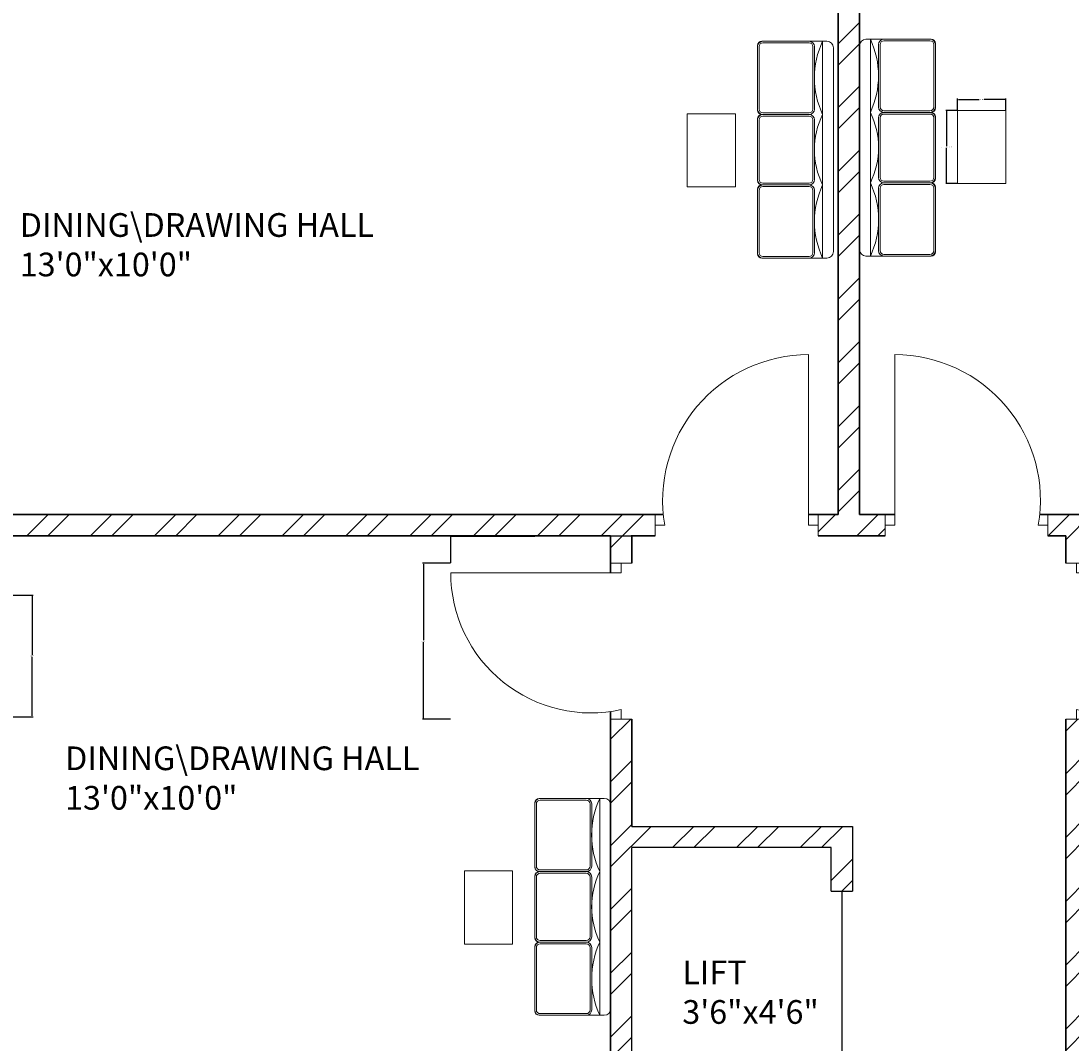
# Model space of a CAD drawing. Units: inches. Extents: x 2165 to 3042, y 1626 to 2968.
# Tile 4 of 11: x 2411 to 2633, y 1996 to 2211. Entities that reach past the tile are written whole.
import ezdxf

# ---------------------------------------------------------------- set-up
doc = ezdxf.new("R2010")
doc.units = ezdxf.units.IN
for name, color, linetype, lineweight in [('A-ANNO-DIMS', 2, 'Continuous', 18), ('A-AREA-IDEN', 7, 'Continuous', 18), ('A-DOOR', 3, 'Continuous', 18), ('A-FLOR-EVTR', 7, 'Continuous', 25), ('A-FURN', 8, 'Continuous', 13), ('A-WALL', 7, 'Continuous', 35), ('A-WALL-PATT', 252, 'Continuous', 13)]:
    doc.layers.add(name, color=color, linetype=linetype, lineweight=lineweight)
doc.styles.get("Standard").update_dxf_attribs({"font": 'arial.ttf'})
doc.dimstyles.get("Standard").update_dxf_attribs({"dimtxt": 0.18, "dimasz": 0.18, "dimexe": 0.18, "dimexo": 0.0625, "dimgap": 0.09, "dimtad": 0, "dimtih": 1, "dimtoh": 1, "dimdec": 4, "dimzin": 0, "dimdsep": 46, "dimtxsty": 'Standard', "dimcen": 0.09, "dimadec": 0, "dimazin": 0, "dimtfac": 1, "dimtdec": 4, "dimtofl": 0, "dimtmove": 0, "dimatfit": 3, "dimfxl": 1, "dimtolj": 1, "dimtzin": 0, "dimarcsym": 0})

# ---------------------------------------------------------------- blocks, each defined once
blk = doc.blocks.new('TABLE-COFFEE')
blk.add_lwpolyline([(0, 15.45), (10.17, 15.45), (10.17, 0), (0, 0)], close=True)
blk = doc.blocks.new('DOOR-36-ENTRY')
for p, q in [((38.25, 32.9), (33.75, 32.9)), ((36, 32.9), (36, 30.9)), ((36, 30.9), (0, 30.9)), ((33.75, 0), (38.25, 0)), ((36, 0), (36, 2))]:
    blk.add_line(p, q)
blk.add_arc((29.6, 30.9), 29.6, 180, 282.4902)
blk = doc.blocks.new('*D22')
at = {"layer": 'A-ANNO-DIMS', "color": 0, "lineweight": -2, "transparency": 16777216}
for p, q in [((2608.74, 2192.37), (2606.31, 2192.37)), ((2606.49, 2192.19), (2606.49, 2184.83)), ((2606.49, 2177.1), (2606.49, 2184.46)), ((2608.74, 2176.92), (2606.31, 2176.92))]:
    blk.add_line(p, q, dxfattribs=at)
at = {"layer": 'A-ANNO-DIMS', "color": 0, "transparency": 16777216}
for points in [[(2606.46, 2192.19), (2606.52, 2192.19), (2606.49, 2192.37)], [(2606.46, 2177.1), (2606.52, 2177.1), (2606.49, 2176.92)]]:
    blk.add_solid(points, dxfattribs=at)
at = {"layer": 'Defpoints', "color": 0, "transparency": 16777216}
for p in [(2608.8, 2192.37), (2606.49, 2176.92), (2608.8, 2176.92)]:
    blk.add_point(p, dxfattribs=at)
at = {"layer": 'A-ANNO-DIMS', "color": 0, "transparency": 16777216, "insert": (2606.49, 2184.65), "char_height": 0.18, "attachment_point": 5}
blk.add_mtext('\\A1;COFFEE TABLE 15 TYP.', dxfattribs=at)
blk = doc.blocks.new('*D23')
at = {"layer": 'A-ANNO-DIMS', "color": 0, "lineweight": -2, "transparency": 16777216}
for p, q in [((2608.8, 2192.44), (2608.8, 2194.87)), ((2608.98, 2194.69), (2613.37, 2194.69)), ((2618.79, 2194.69), (2614.41, 2194.69)), ((2618.97, 2192.44), (2618.97, 2194.87))]:
    blk.add_line(p, q, dxfattribs=at)
at = {"layer": 'A-ANNO-DIMS', "color": 0, "transparency": 16777216}
for points in [[(2608.98, 2194.72), (2608.98, 2194.66), (2608.8, 2194.69)], [(2618.79, 2194.72), (2618.79, 2194.66), (2618.97, 2194.69)]]:
    blk.add_solid(points, dxfattribs=at)
at = {"layer": 'Defpoints', "color": 0, "transparency": 16777216}
for p in [(2608.8, 2194.69), (2608.8, 2192.37), (2618.97, 2192.37)]:
    blk.add_point(p, dxfattribs=at)
at = {"layer": 'A-ANNO-DIMS', "color": 0, "transparency": 16777216, "insert": (2613.89, 2194.69), "char_height": 0.18, "attachment_point": 5}
blk.add_mtext('\\A1;10 TYP.', dxfattribs=at)
blk = doc.blocks.new('*D31')
at = {"layer": 'A-ANNO-DIMS', "color": 0, "lineweight": -2, "transparency": 16777216}
for p, q in [((2408.92, 2090.09), (2413.76, 2090.09)), ((2413.58, 2089.91), (2413.58, 2077.44)), ((2413.58, 2064.6), (2413.58, 2077.08)), ((2408.92, 2064.42), (2413.76, 2064.42))]:
    blk.add_line(p, q, dxfattribs=at)
at = {"layer": 'A-ANNO-DIMS', "color": 0, "transparency": 16777216}
for points in [[(2413.55, 2089.91), (2413.61, 2089.91), (2413.58, 2090.09)], [(2413.55, 2064.6), (2413.61, 2064.6), (2413.58, 2064.42)]]:
    blk.add_solid(points, dxfattribs=at)
at = {"layer": 'Defpoints', "color": 0, "transparency": 16777216}
for p in [(2408.86, 2090.09), (2413.58, 2090.09), (2408.86, 2064.42)]:
    blk.add_point(p, dxfattribs=at)
at = {"layer": 'A-ANNO-DIMS', "color": 0, "transparency": 16777216, "insert": (2413.58, 2077.26), "char_height": 0.18, "attachment_point": 5}
blk.add_mtext('\\A1;26 TYP.', dxfattribs=at)
blk = doc.blocks.new('*D32')
at = {"layer": 'A-ANNO-DIMS', "color": 0, "lineweight": -2, "transparency": 16777216}
for p, q in [((2501.85, 2096.87), (2501.85, 2102.72)), ((2502.03, 2102.54), (2519.58, 2102.54)), ((2539.92, 2102.54), (2522.38, 2102.54)), ((2540.1, 2096.87), (2540.1, 2102.72))]:
    blk.add_line(p, q, dxfattribs=at)
at = {"layer": 'A-ANNO-DIMS', "color": 0, "transparency": 16777216}
for points in [[(2502.03, 2102.57), (2502.03, 2102.51), (2501.85, 2102.54)], [(2539.92, 2102.57), (2539.92, 2102.51), (2540.1, 2102.54)]]:
    blk.add_solid(points, dxfattribs=at)
at = {"layer": 'Defpoints', "color": 0, "transparency": 16777216}
for p in [(2540.1, 2102.54), (2501.85, 2096.8), (2540.1, 2096.8)]:
    blk.add_point(p, dxfattribs=at)
at = {"layer": 'A-ANNO-DIMS', "color": 0, "transparency": 16777216, "insert": (2520.98, 2102.54), "char_height": 0.18, "attachment_point": 5}
blk.add_mtext('\\A1;ENTRY DOOR 38 TYP.', dxfattribs=at)
blk = doc.blocks.new('*D33')
at = {"layer": 'A-ANNO-DIMS', "color": 0, "lineweight": -2, "transparency": 16777216}
for p, q in [((2501.79, 2096.8), (2495.94, 2096.8)), ((2496.12, 2096.62), (2496.12, 2080.54)), ((2496.12, 2064.09), (2496.12, 2080.17)), ((2501.79, 2063.91), (2495.94, 2063.91))]:
    blk.add_line(p, q, dxfattribs=at)
at = {"layer": 'A-ANNO-DIMS', "color": 0, "transparency": 16777216}
for points in [[(2496.09, 2096.62), (2496.15, 2096.62), (2496.12, 2096.8)], [(2496.09, 2064.09), (2496.15, 2064.09), (2496.12, 2063.91)]]:
    blk.add_solid(points, dxfattribs=at)
at = {"layer": 'Defpoints', "color": 0, "transparency": 16777216}
for p in [(2496.12, 2096.8), (2501.85, 2096.8), (2501.85, 2063.91)]:
    blk.add_point(p, dxfattribs=at)
at = {"layer": 'A-ANNO-DIMS', "color": 0, "transparency": 16777216, "insert": (2496.12, 2080.36), "char_height": 0.18, "attachment_point": 5}
blk.add_mtext('\\A1;33 TYP.', dxfattribs=at)
blk = doc.blocks.new('*D51')
at = {"layer": 'A-ANNO-DIMS', "color": 0, "lineweight": -2, "transparency": 16777216}
for p, q in [((2387.04, 2363.58), (2252.12, 2363.58)), ((2252.3, 2363.4), (2252.3, 2082.76)), ((2252.3, 1801.76), (2252.3, 2082.4)), ((2535.54, 1801.58), (2252.12, 1801.58))]:
    blk.add_line(p, q, dxfattribs=at)
at = {"layer": 'A-ANNO-DIMS', "color": 0, "transparency": 16777216}
for points in [[(2252.27, 2363.4), (2252.33, 2363.4), (2252.3, 2363.58)], [(2252.27, 1801.76), (2252.33, 1801.76), (2252.3, 1801.58)]]:
    blk.add_solid(points, dxfattribs=at)
at = {"layer": 'Defpoints', "color": 0, "transparency": 16777216}
for p in [(2252.3, 2363.58), (2387.1, 2363.58), (2535.6, 1801.58)]:
    blk.add_point(p, dxfattribs=at)
at = {"layer": 'A-ANNO-DIMS', "color": 0, "transparency": 16777216, "insert": (2252.3, 2082.58), "char_height": 0.18, "attachment_point": 5}
blk.add_mtext('\\A1;562', dxfattribs=at)

msp = doc.modelspace()

# ---------------------------------------------------------------- hatches: boundary and pattern name
at = {"layer": 'A-WALL-PATT'}
h = msp.add_hatch(dxfattribs=at)
h.set_pattern_fill('ANSI32', color=256)
h.paths.add_polyline_path([(2406.4931, 2332.0783), (2286.6045, 2332.0783), (2286.6045, 2310.967), (2288.8545, 2310.967), (2291.1045, 2310.967), (2291.1045, 2327.5783), (2406.4931, 2327.5783), (2406.4931, 2329.8283)])
h.paths.add_polyline_path([(2439.6045, 2327.5783), (2444.9584, 2327.5783), (2444.9584, 2332.0783), (2430.2901, 2332.0783), (2430.2901, 2329.8283), (2430.2901, 2327.5783), (2435.1045, 2327.5783), (2435.1045, 2219.5783), (2431.0902, 2219.5783), (2431.0902, 2215.0783), (2435.1045, 2215.0783), (2444.1108, 2215.0783), (2444.1108, 2217.3283), (2444.1108, 2219.5783), (2439.6045, 2219.5783)])
h.paths.add_polyline_path([(2497.5418, 2329.8283), (2497.5418, 2332.0783), (2470.1978, 2332.0783), (2470.1978, 2327.5783), (2497.5418, 2327.5783)])
h.paths.add_polyline_path([(2617.9543, 2332.0783), (2557.5418, 2332.0783), (2557.5418, 2327.5783), (2583.6045, 2327.5783), (2583.6045, 2219.5783), (2474.0523, 2219.5783), (2474.0523, 2215.0783), (2583.6045, 2215.0783), (2583.6045, 2107.0783), (2579.3609, 2107.0783), (2579.3609, 2102.5783), (2588.1045, 2102.5783), (2593.5283, 2102.5783), (2593.5283, 2104.8283), (2593.5283, 2107.0783), (2588.1045, 2107.0783), (2588.1045, 2215.0783), (2691.2325, 2215.0783), (2691.2325, 2217.3283), (2691.2325, 2219.5783), (2588.1045, 2219.5783), (2588.1045, 2327.5783), (2617.9543, 2327.5783)])
h.paths.add_polyline_path([(2702.4444, 2329.8283), (2702.4444, 2332.0783), (2677.9543, 2332.0783), (2677.9543, 2327.5783), (2702.4444, 2327.5783)])
h.paths.add_polyline_path([(2736.6045, 2327.5783), (2742.5161, 2327.5783), (2742.5161, 2329.8283), (2742.5161, 2332.0783), (2727.7639, 2332.0783), (2727.7639, 2329.8283), (2727.7639, 2327.5783), (2732.1045, 2327.5783), (2732.1045, 2219.5783), (2726.4404, 2219.5783), (2726.4404, 2215.0783), (2732.1045, 2215.0783), (2742.7291, 2215.0783), (2742.7291, 2217.3283), (2742.7291, 2219.5783), (2736.6045, 2219.5783)])
h.paths.add_polyline_path([(2885.1045, 2332.0783), (2768.4887, 2332.0783), (2768.4887, 2327.5783), (2784.6045, 2327.5783), (2880.6045, 2327.5783), (2880.6045, 2310.967), (2885.1045, 2310.967)])
h.paths.add_polyline_path([(2885.1045, 2250.967), (2880.6045, 2250.967), (2880.6045, 2219.5783), (2776.5755, 2219.5783), (2776.5755, 2215.0783), (2788.1045, 2215.0783), (2788.1045, 2209.8634), (2790.3545, 2209.8634), (2792.6045, 2209.8634), (2792.6045, 2215.0783), (2880.6045, 2215.0783), (2880.6045, 2139.0783), (2871.2037, 2139.0783), (2871.2037, 2134.5783), (2885.1045, 2134.5783)])
h.paths.add_polyline_path([(2545.013, 2107.0783), (2474.0523, 2107.0783), (2291.1045, 2107.0783), (2291.1045, 2102.5783), (2535.6045, 2102.5783), (2535.6045, 2096.8046), (2537.8545, 2096.8046), (2540.1045, 2096.8046), (2540.1045, 2102.5783), (2545.013, 2102.5783), (2545.013, 2104.8283)])
h.paths.add_polyline_path([(2397.7297, 2217.3283), (2397.7297, 2219.5783), (2291.1045, 2219.5783), (2291.1045, 2250.967), (2286.6045, 2250.967), (2286.6045, 2206.1346), (2288.8545, 2206.1346), (2291.1045, 2206.1346), (2291.1045, 2215.0783), (2367.1045, 2215.0783), (2367.1045, 2212.2868), (2371.6045, 2212.2868), (2371.6045, 2215.0783), (2397.7297, 2215.0783)])
h.paths.add_polyline_path([(2291.1045, 1978.5783), (2367.1045, 1978.5783), (2371.6045, 1978.5783), (2373.2641, 1978.5783), (2374.4883, 1978.5783), (2374.4883, 1980.8283), (2374.4883, 1983.0783), (2371.6045, 1983.0783), (2371.6045, 1986.964), (2369.9051, 1986.964), (2369.3545, 1986.964), (2367.1045, 1986.964), (2367.1045, 1983.0783), (2291.1045, 1983.0783), (2291.1045, 2001.1808), (2286.6045, 2001.1808), (2286.6045, 1947.0203), (2288.8545, 1947.0203), (2291.1045, 1947.0203)])
h.paths.add_polyline_path([(2291.1045, 1887.0203), (2286.6045, 1887.0203), (2286.6045, 1842.0783), (2381.2561, 1842.0783), (2381.2561, 1844.3283), (2381.2561, 1846.5783), (2363.1045, 1846.5783), (2291.1045, 1846.5783)])
h.paths.add_polyline_path([(2415.6045, 1978.5783), (2421.1681, 1978.5783), (2421.1681, 1983.0783), (2415.6045, 1983.0783), (2406.5227, 1983.0783), (2406.5227, 1980.8283), (2406.5227, 1978.5783), (2411.1045, 1978.5783), (2411.1045, 1846.5783), (2406.7549, 1846.5783), (2406.7549, 1842.0783), (2419.2885, 1842.0783), (2419.2885, 1844.3283), (2419.2885, 1846.5783), (2415.6045, 1846.5783)])
h.paths.add_polyline_path([(2586.6045, 1982.779), (2586.6045, 1991.5911), (2582.1045, 1991.5911), (2582.1045, 1982.779), (2540.1045, 1982.779), (2540.1045, 2036.779), (2582.1045, 2036.779), (2582.1045, 2027.6051), (2586.6045, 2027.6051), (2586.6045, 2041.279), (2582.1045, 2041.279), (2540.1045, 2041.279), (2540.1045, 2063.9064), (2537.8545, 2063.9064), (2535.6045, 2063.9064), (2535.6045, 1983.0783), (2455.068, 1983.0783), (2455.068, 1978.5783), (2535.6045, 1978.5783), (2535.6045, 1846.5783), (2522.622, 1846.5783), (2522.622, 1842.0783), (2535.6045, 1842.0783), (2535.6045, 1806.0783), (2535.6045, 1801.5783), (2556.726, 1801.5783), (2556.726, 1803.8283), (2556.726, 1806.0783), (2540.1045, 1806.0783), (2540.1045, 1842.0783), (2540.1045, 1846.5783), (2540.1045, 1978.279), (2586.6045, 1978.279)])
h.paths.add_polyline_path([(2636.1045, 1978.5783), (2717.6642, 1978.5783), (2717.6642, 1980.8283), (2717.6642, 1983.0783), (2636.1045, 1983.0783), (2636.1045, 2063.9064), (2633.8545, 2063.9064), (2631.6045, 2063.9064), (2631.6045, 1846.5783), (2631.6045, 1842.0783), (2631.6045, 1806.0783), (2604.726, 1806.0783), (2604.726, 1801.5783), (2636.1045, 1801.5783), (2636.1045, 1842.0783), (2644.3411, 1842.0783), (2644.3411, 1844.3283), (2644.3411, 1846.5783), (2636.1045, 1846.5783)])
h.paths.add_polyline_path([(2760.6045, 1978.5783), (2764.9931, 1978.5783), (2764.9931, 1983.0783), (2750.4727, 1983.0783), (2750.4727, 1980.8283), (2750.4727, 1978.5783), (2756.1045, 1978.5783), (2756.1045, 1846.5783), (2749.4543, 1846.5783), (2749.4543, 1842.0783), (2765.1894, 1842.0783), (2765.1894, 1846.5783), (2760.6045, 1846.5783)])
h.paths.add_polyline_path([(2880.6045, 1983.0783), (2804.6045, 1983.0783), (2804.6045, 1988.3825), (2802.3545, 1988.3825), (2800.1045, 1988.3825), (2800.1045, 1983.0783), (2800.1045, 1978.5783), (2880.6045, 1978.5783)])
h.paths.add_polyline_path([(2885.1045, 2075.5783), (2871.2037, 2075.5783), (2871.2037, 2071.0783), (2880.6045, 2071.0783), (2880.6045, 1948.8144), (2885.1045, 1948.8144)])
h.paths.add_polyline_path([(2885.1045, 1888.8144), (2880.6045, 1888.8144), (2880.6045, 1846.5783), (2792.1167, 1846.5783), (2792.1167, 1842.0783), (2885.1045, 1842.0783)])
h.paths.add_polyline_path([(2724.4848, 1846.5783), (2708.1045, 1846.5783), (2692.3411, 1846.5783), (2692.3411, 1842.0783), (2724.4848, 1842.0783), (2724.4848, 1844.3283)])
h.paths.add_polyline_path([(2474.622, 1844.4672), (2474.622, 1846.5783), (2444.7417, 1846.5783), (2444.7417, 1842.0783), (2474.622, 1842.0783)])
h = msp.add_hatch(dxfattribs=at)
h.set_pattern_fill('ANSI32', color=256)
h.paths.add_polyline_path([(2834.3545, 2109.2607), (2832.1045, 2109.2607), (2829.8545, 2109.2607), (2829.8545, 2107.0783), (2788.1045, 2107.0783), (2627.8367, 2107.0783), (2627.8367, 2102.5783), (2631.6045, 2102.5783), (2631.6045, 2096.8046), (2636.1045, 2096.8046), (2636.1045, 2102.5783), (2788.1045, 2102.5783), (2829.8545, 2102.5783), (2829.8545, 2099.5599), (2834.3545, 2099.5599), (2834.3545, 2102.5783)])
h.paths.add_polyline_path([(2834.3545, 2162.7002), (2834.3545, 2167.2002), (2792.6045, 2167.2002), (2792.6045, 2188.8893), (2790.3545, 2188.8893), (2788.1045, 2188.8893), (2788.1045, 2162.7002), (2829.8545, 2162.7002), (2829.8545, 2134.5783), (2829.8545, 2129.9534), (2834.3545, 2129.9534), (2834.3545, 2134.5783), (2847.2037, 2134.5783), (2847.2037, 2139.0783), (2834.3545, 2139.0783)])
h.paths.add_polyline_path([(2834.3545, 2071.0783), (2847.2037, 2071.0783), (2847.2037, 2075.5783), (2834.3545, 2075.5783), (2834.3545, 2078.8214), (2829.8545, 2078.8214), (2829.8545, 2075.5783), (2829.8545, 2034.1177), (2800.1045, 2034.1177), (2800.1045, 2011.8162), (2802.3375, 2011.8162), (2804.6045, 2011.8162), (2804.6045, 2029.6177), (2834.3545, 2029.6177), (2834.3545, 2034.1177)])

# ---------------------------------------------------------------- linework, layer by layer
at = {"layer": 'A-DOOR'}
for p, q in [((2577.3609, 2104.8283), (2577.3609, 2140.8283)), ((2595.5283, 2104.8283), (2595.5283, 2140.8283)), ((2545.013, 2107.0783), (2545.013, 2102.5783)), ((2579.3609, 2107.0783), (2579.3609, 2102.5783)), ((2593.5283, 2107.0783), (2593.5283, 2102.5783)), ((2627.8367, 2107.0783), (2627.8367, 2102.5783)), ((2545.013, 2102.5783), (2545.013, 2104.8283)), ((2545.013, 2104.8283), (2547.013, 2104.8283)), ((2579.3609, 2104.8283), (2577.3609, 2104.8283)), ((2579.3609, 2102.5783), (2579.3609, 2104.8283)), ((2593.5283, 2102.5783), (2593.5283, 2104.8283)), ((2593.5283, 2104.8283), (2595.5283, 2104.8283)), ((2627.8367, 2104.8283), (2625.8367, 2104.8283)), ((2627.8367, 2102.5783), (2627.8367, 2104.8283)), ((2535.6045, 2096.8046), (2537.8545, 2096.8046)), ((2540.1045, 2063.9064), (2537.8545, 2063.9064))]:
    msp.add_line(p, q, dxfattribs=at)
for centre, radius, start, end in [((2577.3609, 2110.0367), 30.7916, 90, 189.738379), ((2595.5283, 2110.07), 30.7583, 350.18795, 90)]:
    msp.add_arc(centre, radius, start, end, dxfattribs=at)
at = {"layer": 'A-FLOR-EVTR'}
for p, q in [((2540.1045, 2041.279), (2582.1045, 2041.279)), ((2582.1045, 2041.279), (2586.6045, 2041.279)), ((2586.6045, 2041.279), (2586.6045, 2027.6051)), ((2582.1045, 2036.779), (2540.1045, 2036.779)), ((2540.1045, 1982.779), (2540.1045, 2036.779)), ((2582.1045, 2027.6051), (2582.1045, 2036.779)), ((2582.1045, 2027.6051), (2586.6045, 2027.6051)), ((2584.3545, 2027.6051), (2584.3545, 1991.5911))]:
    msp.add_line(p, q, dxfattribs=at)
at = {"layer": 'A-FURN'}
for points in [[(2567.7416, 2191.5179), (2577.4675, 2191.5179, 0.41421356), (2578.6117, 2192.6621), (2578.6117, 2205.8207, 0.41421356), (2577.4675, 2206.9649), (2567.7416, 2206.9649, 0.41421356), (2566.5974, 2205.8207), (2566.5974, 2192.6621, 0.41421356)], [(2567.7416, 2191.8612), (2577.4675, 2191.8612, 0.41421356), (2578.2684, 2192.6621), (2578.2684, 2205.8207, 0.41421356), (2577.4675, 2206.6216), (2567.7416, 2206.6216, 0.41421356), (2566.9406, 2205.8207), (2566.9406, 2192.6621, 0.41421356)], [(2602.9794, 2207.3978), (2593.2535, 2207.3978, 0.41421356), (2592.1092, 2206.2536), (2592.1092, 2193.095, 0.41421356), (2593.2535, 2191.9508), (2602.9794, 2191.9508, 0.41421356), (2604.1236, 2193.095), (2604.1236, 2206.2536, 0.41421356)], [(2602.9794, 2207.0545), (2593.2535, 2207.0545, 0.41421356), (2592.4525, 2206.2536), (2592.4525, 2193.095, 0.41421356), (2593.2535, 2192.294), (2602.9794, 2192.294, 0.41421356), (2603.7803, 2193.095), (2603.7803, 2206.2536, 0.41421356)], [(2567.7416, 2191.5179), (2577.4675, 2191.5179, -0.41421356), (2578.6117, 2190.3737), (2578.6117, 2177.7872, -0.41421356), (2577.4675, 2176.643), (2567.7416, 2176.643, -0.41421356), (2566.5974, 2177.7872), (2566.5974, 2190.3737, -0.41421356)], [(2567.7416, 2191.1746), (2577.4675, 2191.1746, -0.41421356), (2578.2684, 2190.3737), (2578.2684, 2177.7872, -0.41421356), (2577.4675, 2176.9863), (2567.7416, 2176.9863, -0.41421356), (2566.9406, 2177.7872), (2566.9406, 2190.3737, -0.41421356)], [(2602.9794, 2177.0759), (2593.2535, 2177.0759, -0.41421356), (2592.1092, 2178.2201), (2592.1092, 2190.8066, -0.41421356), (2593.2535, 2191.9508), (2602.9794, 2191.9508, -0.41421356), (2604.1236, 2190.8066), (2604.1236, 2178.2201, -0.41421356)], [(2602.9794, 2177.4191), (2593.2535, 2177.4191, -0.41421356), (2592.4525, 2178.2201), (2592.4525, 2190.8066, -0.41421356), (2593.2535, 2191.6075), (2602.9794, 2191.6075, -0.41421356), (2603.7803, 2190.8066), (2603.7803, 2178.2201, -0.41421356)], [(2567.7416, 2161.196), (2577.4675, 2161.196, 0.41421356), (2578.6117, 2162.3402), (2578.6117, 2175.4988, 0.41421356), (2577.4675, 2176.643), (2567.7416, 2176.643, 0.41421356), (2566.5974, 2175.4988), (2566.5974, 2162.3402, 0.41421356)], [(2567.7416, 2161.5392), (2577.4675, 2161.5392, 0.41421356), (2578.2684, 2162.3402), (2578.2684, 2175.4988, 0.41421356), (2577.4675, 2176.2997), (2567.7416, 2176.2997, 0.41421356), (2566.9406, 2175.4988), (2566.9406, 2162.3402, 0.41421356)], [(2602.9794, 2177.0759), (2593.2535, 2177.0759, 0.41421356), (2592.1092, 2175.9316), (2592.1092, 2162.7731, 0.41421356), (2593.2535, 2161.6289), (2602.9794, 2161.6289, 0.41421356), (2604.1236, 2162.7731), (2604.1236, 2175.9316, 0.41421356)], [(2602.9794, 2176.7326), (2593.2535, 2176.7326, 0.41421356), (2592.4525, 2175.9316), (2592.4525, 2162.7731, 0.41421356), (2593.2535, 2161.9721), (2602.9794, 2161.9721, 0.41421356), (2603.7803, 2162.7731), (2603.7803, 2175.9316, 0.41421356)], [(2520.7295, 2031.7259), (2530.4554, 2031.7259, 0.41421356), (2531.5997, 2032.8701), (2531.5997, 2046.0286, 0.41421356), (2530.4554, 2047.1729), (2520.7295, 2047.1729, 0.41421356), (2519.5853, 2046.0286), (2519.5853, 2032.8701, 0.41421356)], [(2520.7295, 2032.0691), (2530.4554, 2032.0691, 0.41421356), (2531.2564, 2032.8701), (2531.2564, 2046.0286, 0.41421356), (2530.4554, 2046.8296), (2520.7295, 2046.8296, 0.41421356), (2519.9286, 2046.0286), (2519.9286, 2032.8701, 0.41421356)], [(2520.7295, 2031.7259), (2530.4554, 2031.7259, -0.41421356), (2531.5997, 2030.5816), (2531.5997, 2017.9952, -0.41421356), (2530.4554, 2016.8509), (2520.7295, 2016.8509, -0.41421356), (2519.5853, 2017.9952), (2519.5853, 2030.5816, -0.41421356)], [(2520.7295, 2031.3826), (2530.4554, 2031.3826, -0.41421356), (2531.2564, 2030.5816), (2531.2564, 2017.9952, -0.41421356), (2530.4554, 2017.1942), (2520.7295, 2017.1942, -0.41421356), (2519.9286, 2017.9952), (2519.9286, 2030.5816, -0.41421356)], [(2520.7295, 2001.4039), (2530.4554, 2001.4039, 0.41421356), (2531.5997, 2002.5482), (2531.5997, 2015.7067, 0.41421356), (2530.4554, 2016.8509), (2520.7295, 2016.8509, 0.41421356), (2519.5853, 2015.7067), (2519.5853, 2002.5482, 0.41421356)], [(2520.7295, 2001.7472), (2530.4554, 2001.7472, 0.41421356), (2531.2564, 2002.5482), (2531.2564, 2015.7067, 0.41421356), (2530.4554, 2016.5077), (2520.7295, 2016.5077, 0.41421356), (2519.9286, 2015.7067), (2519.9286, 2002.5482, 0.41421356)]]:
    msp.add_lwpolyline(points, format="xyb", close=True, dxfattribs=at)
at = {"layer": 'A-FURN', "ltscale": 0.03}
for points in [[(2566.5974, 2175.7164), (2566.5974, 2162.1114, 0.41421356), (2567.5127, 2161.196), (2581.2434, 2161.196, 0.41421356), (2582.6165, 2162.569), (2582.6165, 2205.5918, 0.41421356), (2581.2434, 2206.9649), (2567.5127, 2206.9649, 0.41421356), (2566.5974, 2206.0495), (2566.5974, 2192.4445, 0.41421356), (2567.5127, 2191.5291, -1), (2567.5127, 2191.5066, 0.41421356), (2566.5974, 2190.5913), (2566.5974, 2177.5696, 0.41421356), (2567.5127, 2176.6542, -1), (2567.5127, 2176.6317, 0.41421356)], [(2604.1236, 2192.8774), (2604.1236, 2206.4824, 0.41421356), (2603.2082, 2207.3978), (2589.4775, 2207.3978, 0.41421356), (2588.1045, 2206.0247), (2588.1045, 2163.0019, 0.41421356), (2589.4775, 2161.6289), (2603.2082, 2161.6289, 0.41421356), (2604.1236, 2162.5442), (2604.1236, 2176.1492, 0.41421356), (2603.2082, 2177.0646, -1), (2603.2082, 2177.0871, 0.41421356), (2604.1236, 2178.0025), (2604.1236, 2191.0241, 0.41421356), (2603.2082, 2191.9395, -1), (2603.2082, 2191.962, 0.41421356)], [(2519.5853, 2015.9243), (2519.5853, 2002.3193, 0.41421356), (2520.5007, 2001.4039), (2534.2314, 2001.4039, 0.41421356), (2535.6045, 2002.777), (2535.6045, 2045.7998, 0.41421356), (2534.2314, 2047.1729), (2520.5007, 2047.1729, 0.41421356), (2519.5853, 2046.2575), (2519.5853, 2032.6525, 0.41421356), (2520.5007, 2031.7371, -1), (2520.5007, 2031.7146, 0.41421356), (2519.5853, 2030.7992), (2519.5853, 2017.7776, 0.41421356), (2520.5007, 2016.8622, -1), (2520.5007, 2016.8397, 0.41421356)]]:
    msp.add_lwpolyline(points, format="xyb", close=True, dxfattribs=at)
at = {"layer": 'A-FURN'}
for points in [[(2580.3281, 2161.196), (2580.3281, 2206.9649)], [(2590.3929, 2207.3978), (2590.3929, 2161.6289)], [(2533.316, 2001.4039), (2533.316, 2047.1729)]]:
    msp.add_lwpolyline(points, dxfattribs=at)
for centre, radius, start, end in [((2596.6332, 2199.2414), 18.0419, 154.653824, 205.346176), ((2573.897, 2199.6743), 18.2145, 334.910626, 25.089374), ((2595.489, 2184.0804), 16.887, 153.868999, 206.131001), ((2575.2319, 2184.5133), 16.887, 333.868999, 26.131001), ((2596.8239, 2168.9195), 18.2145, 154.910626, 205.089374), ((2574.0877, 2169.3524), 18.0419, 334.653824, 25.346176), ((2549.6212, 2039.4494), 18.0419, 154.653824, 205.346176), ((2548.477, 2024.2884), 16.887, 153.868999, 206.131001), ((2549.8119, 2009.1274), 18.2145, 154.910626, 205.089374)]:
    msp.add_arc(centre, radius, start, end, dxfattribs=at)
at = {"layer": 'A-WALL'}
for p, q in [((2583.6045, 2215.0783), (2583.6045, 2107.0783)), ((2588.1045, 2215.0783), (2588.1045, 2107.0783)), ((2291.1045, 2107.0783), (2546.7118, 2107.0783)), ((2474.0523, 2107.0783), (2546.7118, 2107.0783)), ((2577.3609, 2107.0783), (2583.6045, 2107.0783)), ((2577.3609, 2107.0783), (2583.6045, 2107.0783)), ((2588.1045, 2107.0783), (2595.5283, 2107.0783)), ((2626.1408, 2107.0783), (2788.1045, 2107.0783)), ((2291.1045, 2102.5783), (2535.6045, 2102.5783)), ((2474.0523, 2102.5783), (2535.6045, 2102.5783)), ((2535.6045, 2094.8046), (2535.6045, 2102.5783)), ((2540.1045, 2096.8046), (2540.1045, 2102.5783)), ((2540.1045, 2102.5783), (2545.013, 2102.5783)), ((2540.1045, 2102.5783), (2545.013, 2102.5783)), ((2579.3609, 2102.5783), (2588.1045, 2102.5783)), ((2579.3609, 2102.5783), (2588.1045, 2102.5783)), ((2588.1045, 2102.5783), (2593.5283, 2102.5783)), ((2627.8367, 2102.5783), (2631.6045, 2102.5783)), ((2631.6045, 2102.5783), (2631.6045, 2096.8046)), ((2535.6045, 1983.0783), (2535.6045, 2065.4985)), ((2540.1045, 2041.279), (2540.1045, 2063.9064)), ((2631.6045, 2063.9064), (2631.6045, 1846.5783))]:
    msp.add_line(p, q, dxfattribs=at)

# ---------------------------------------------------------------- block references
at = {"layer": 'A-DOOR'}
msp.add_blockref('DOOR-36-ENTRY', (2501.854, 2063.906), dxfattribs=at)
at = {"layer": 'A-DOOR', "extrusion": (0, 0, -1), "zscale": -1}
msp.add_blockref('DOOR-36-ENTRY', (-2669.8549, 2063.906), dxfattribs=at)
at = {"layer": 'A-FURN'}
for p in [(2551.752, 2176.221), (2504.74, 2016.429)]:
    msp.add_blockref('TABLE-COFFEE', p, dxfattribs=at)
at = {"layer": 'A-FURN', "rotation": 180}
msp.add_blockref('TABLE-COFFEE', (2618.9689, 2192.3728), dxfattribs=at)

# ---------------------------------------------------------------- texts
at = {"layer": 'A-AREA-IDEN', "char_height": 5, "attachment_point": 1}
for s, width, insert in [('DINING\\\\DRAWING HALL\\P13\'0"x10\'0"', 87.849088, (2410.9185, 2170.6864)), ('DINING\\\\DRAWING HALL\\P13\'0"x10\'0"', 148.447573, (2420.4947, 2058.1363)), ('LIFT\\P3\'6"x4\'6"', 73.014705, (2550.7198, 2012.9421))]:
    msp.add_mtext_dynamic_manual_height_columns(s, width=width, gutter_width=12.5, heights=[0], dxfattribs=dict(at, insert=insert))

# ---------------------------------------------------------------- dimensions: what is measured, and where the dimension line sits
at = {"layer": 'A-ANNO-DIMS'}
dim = msp.add_linear_dim(base=(2252.3045, 2363.5783), p1=(2535.6045, 1801.5783), p2=(2387.1045, 2363.5783), angle=90, dimstyle='Standard', override={"dimdec": 0, "dimlfac": 1, "dimrnd": 0, "dimzin": 0, "dimdsep": 46, "dimlunit": 2}, dxfattribs=at)
dim.commit()
dim.dimension.update_dxf_attribs({"geometry": '*D51', "text_midpoint": (2252.3045, 2082.5783)})
for base, p1, p2, angle, text, picture, middle in [((2608.8026, 2194.6901), (2618.9692, 2192.3725), (2608.8026, 2192.3725), 180, '<> TYP.', '*D23', (2613.8859, 2194.6901)), ((2606.485, 2176.9223), (2608.8026, 2192.3725), (2608.8026, 2176.9223), 270, 'COFFEE TABLE <> TYP.', '*D22', (2606.485, 2184.6474)), ((2496.117, 2096.8046), (2501.8545, 2063.9064), (2501.8545, 2096.8046), 90, '<> TYP.', '*D33', (2496.117, 2080.3555)), ((2413.579, 2090.0947), (2408.8594, 2064.4239), (2408.8594, 2090.0947), 90, '<> TYP.', '*D31', (2413.579, 2077.2593))]:
    dim = msp.add_linear_dim(base=base, p1=p1, p2=p2, angle=angle, text=text, dimstyle='Standard', override={"dimdec": 0, "dimlfac": 1, "dimrnd": 0, "dimzin": 0, "dimdsep": 46, "dimlunit": 2}, dxfattribs=at)
    dim.commit()
    dim.dimension.update_dxf_attribs({"geometry": picture, "text_midpoint": middle})
dim = msp.add_linear_dim(base=(2540.1045, 2102.5421), p1=(2501.8545, 2096.8046), p2=(2540.1045, 2096.8046), text='ENTRY DOOR <> TYP.', dimstyle='Standard', override={"dimdec": 0, "dimlfac": 1, "dimrnd": 0, "dimzin": 0, "dimdsep": 46, "dimlunit": 2}, dxfattribs=at)
dim.commit()
dim.dimension.update_dxf_attribs({"geometry": '*D32', "text_midpoint": (2520.9795, 2102.5421)})

doc.saveas('drawing.dxf')
